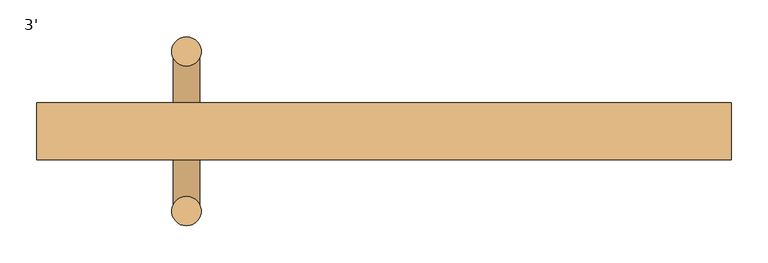
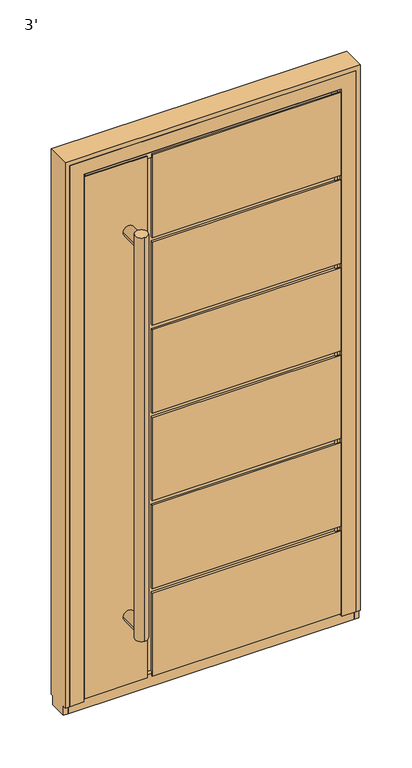
"""IFC4 building model written with IfcOpenShell, lengths in millimetres: door geometry, 3'."""

from ifc_helpers import new_model, si_unit, point, frame, frame_2d, origin, place, context, project, spatial, circle_curve, trimmed, segment, composite_curve, outline, extrude, faceted_brep, source, transform, mapped, element, save


def door_3_44036f4b(model_context):
    return source(origin(), model_context, "Body", "SolidModel", [
        extrude(outline(composite_curve([segment(trimmed(circle_curve(frame_2d((-268.65, 90.8003001)), 20.0), [point((-268.65, 70.8003001))], [point((-268.65, 110.8003001))], False, "CARTESIAN"), True, "CONTINUOUS"), segment(trimmed(circle_curve(frame_2d((-268.65, 90.8003001)), 20.0), [point((-268.65, 110.8003001))], [point((-268.65, 70.8003001))], False, "CARTESIAN"), True, "CONTINUOUS")], self_intersect=False)), frame((0.0, 0.0, 210.0000003), z_axis=(0.0, 0.0, 1.0), x_axis=(1.0, 0.0, 0.0)), (0.0, 0.0, 1.0), 1363.8),
        extrude(outline(composite_curve([segment(trimmed(circle_curve(frame_2d((-268.65, -126.2003001)), 20.0), [point((-268.65, -146.2003001))], [point((-268.65, -106.2003001))], False, "CARTESIAN"), True, "CONTINUOUS"), segment(trimmed(circle_curve(frame_2d((-268.65, -126.2003001)), 20.0), [point((-268.65, -106.2003001))], [point((-268.65, -146.2003001))], False, "CARTESIAN"), True, "CONTINUOUS")], self_intersect=False)), frame((0.0, 0.0, 210.0000003), z_axis=(0.0, 0.0, 1.0), x_axis=(1.0, 0.0, 0.0)), (0.0, 0.0, 1.0), 1363.8),
        extrude(outline(composite_curve([segment(trimmed(circle_curve(frame_2d((241.9000003, -268.65)), 18.0), [point((241.9000003, -286.65))], [point((241.9000003, -250.65))], False, "CARTESIAN"), True, "CONTINUOUS"), segment(trimmed(circle_curve(frame_2d((241.9000003, -268.65)), 18.0), [point((241.9000003, -250.65))], [point((241.9000003, -286.65))], False, "CARTESIAN"), True, "CONTINUOUS")], self_intersect=False)), frame((0.0, -126.2, 0.0), z_axis=(0.0, 1.0, 0.0), x_axis=(0.0, 0.0, 1.0)), (0.0, 0.0, 1.0), 217.0),
        extrude(outline(composite_curve([segment(trimmed(circle_curve(frame_2d((1541.9000003, -268.65)), 18.0), [point((1541.9000003, -286.65))], [point((1541.9000003, -250.65))], False, "CARTESIAN"), True, "CONTINUOUS"), segment(trimmed(circle_curve(frame_2d((1541.9000003, -268.65)), 18.0), [point((1541.9000003, -250.65))], [point((1541.9000003, -286.65))], False, "CARTESIAN"), True, "CONTINUOUS")], self_intersect=False)), frame((0.0, -126.2, 0.0), z_axis=(0.0, 1.0, 0.0), x_axis=(0.0, 0.0, 1.0)), (0.0, 0.0, 1.0), 217.0),
        faceted_brep([(-193.65, 13.8, 306.466667), (383.65, 13.8, 306.466667), (383.65, 13.8, 291.466667), (-193.65, 13.8, 291.466667), (-193.65, 13.8, 35.0), (-208.65, 13.8, 35.0), (-208.65, 13.8, 1748.8000003), (-193.65, 13.8, 1748.8000003), (-193.65, 13.8, 1492.3333337), (383.65, 13.8, 1492.3333337), (383.65, 13.8, 1477.3333337), (-193.65, 13.8, 1477.3333337), (-193.65, 13.8, 1195.866667), (383.65, 13.8, 1195.866667), (383.65, 13.8, 1180.866667), (-193.65, 13.8, 1180.866667), (-193.65, 13.8, 899.4000004), (383.65, 13.8, 899.4000004), (383.65, 13.8, 884.4000004), (-193.65, 13.8, 884.4000004), (-193.65, 13.8, 602.9333337), (383.65, 13.8, 602.9333337), (383.65, 13.8, 587.9333337), (-193.65, 13.8, 587.9333337), (-193.65, 20.8, 587.9333337), (-193.65, 20.8, 306.466667), (383.65, 20.8, 587.9333337), (383.65, 11.7997698, 1748.8000003), (383.65, 11.7997698, 35.0), (383.65, 18.8020472, 35.0), (383.65, 18.8020472, 24.0), (383.65, 20.8, 24.0), (383.65, 20.8, 291.466667), (383.65, 20.8, 306.466667), (383.65, 20.8, 602.9333337), (383.65, 20.8, 884.4000004), (383.65, 20.8, 899.4000004), (383.65, 20.8, 1180.866667), (383.65, 20.8, 1195.866667), (383.65, 20.8, 1477.3333337), (383.65, 20.8, 1492.3333337), (383.65, 20.8, 1748.8000003), (-193.65, 20.8, 602.9333337), (-193.65, 20.8, 884.4000004), (-193.65, 20.8, 899.4000004), (-193.65, 20.8, 1180.866667), (-208.65, 18.8020472, 35.0), (-208.65, 18.8020472, 24.0), (-208.65, 20.8, 24.0), (-208.65, 20.8, 1748.8000003), (-383.65, 11.7997698, 35.0), (-383.65, 18.8020472, 35.0), (-193.65, 18.8020472, 35.0), (-193.65, 20.8, 291.466667), (-193.65, 20.8, 24.0), (-193.65, 18.8020472, 24.0), (-383.65, 18.8020472, 24.0), (-383.65, 20.8, 24.0), (-383.65, 20.8, 1748.8000003), (-193.65, 20.8, 1195.866667), (-193.65, 20.8, 1477.3333337), (-193.65, 20.8, 1492.3333337), (-193.65, 20.8, 1748.8000003), (408.65, -56.2, 10.0000003), (-193.65, -56.2, 10.0000003), (-193.65, -53.2, 10.0000003), (408.65, -53.2, 10.0000003), (-408.65, -53.2, 10.0000003), (-208.65, -53.2, 10.0000003), (-208.65, -56.2, 10.0000003), (-408.65, -56.2, 10.0000003), (408.65, -56.2, 306.466667), (408.65, -53.2, 306.466667), (408.65, -53.2, 587.9333337), (408.65, -56.2, 587.9333337), (408.65, -56.2, 899.4000004), (408.65, -53.2, 899.4000004), (408.65, -53.2, 1180.866667), (408.65, -56.2, 1180.866667), (408.65, -56.2, 602.9333337), (408.65, -53.2, 602.9333337), (408.65, -53.2, 884.4000004), (408.65, -56.2, 884.4000004), (408.65, -56.2, 1195.866667), (408.65, -53.2, 1195.866667), (408.65, -53.2, 1477.3333337), (408.65, -56.2, 1477.3333337), (408.65, -56.2, 1773.8000003), (408.65, -56.2, 1492.3333337), (408.65, -53.2, 1492.3333337), (408.65, -53.2, 1773.8000003), (408.65, -53.2, 291.466667), (408.65, -56.2, 291.466667), (-193.65, -53.2, 25.5), (393.15, -53.2, 25.5), (393.15, -53.2, 291.466667), (393.15, -53.2, 306.466667), (393.15, -53.2, 587.9333337), (393.15, -53.2, 899.4000004), (393.15, -53.2, 1180.866667), (393.15, -53.2, 602.9333337), (393.15, -53.2, 884.4000004), (-393.15, -53.2, 25.5), (-208.65, -53.2, 25.5), (-408.65, -53.2, 1773.8000003), (-208.65, -53.2, 1773.8000003), (-208.65, -53.2, 1758.3000003), (-393.15, -53.2, 1758.3000003), (393.15, -53.2, 1195.866667), (393.15, -53.2, 1477.3333337), (393.15, -53.2, 1492.3333337), (393.15, -53.2, 1758.3000003), (-193.65, -53.2, 1758.3000003), (-193.65, -53.2, 1773.8000003), (-193.65, -49.2, 291.466667), (-193.65, -49.2, 25.5), (-193.65, -56.2, 291.466667), (-208.65, -56.2, 1773.8000003), (-408.65, -56.2, 1773.8000003), (-193.65, -56.2, 587.9333337), (-193.65, -56.2, 306.466667), (-193.65, -56.2, 1180.866667), (-193.65, -56.2, 899.4000004), (-193.65, -56.2, 884.4000004), (-193.65, -56.2, 602.9333337), (-193.65, -56.2, 1477.3333337), (-193.65, -56.2, 1195.866667), (-193.65, -56.2, 1773.8000003), (-193.65, -56.2, 1492.3333337), (-208.65, -49.2, 1758.3000003), (-208.65, -49.2, 25.5), (-383.65, 11.7997698, 1748.8000003), (393.15, 11.7997698, 1758.3000003), (393.15, 11.7997698, 25.5), (-393.15, 11.7997698, 25.5), (-393.15, 11.7997698, 1758.3000003), (393.15, -49.2, 1492.3333337), (393.15, -49.2, 1477.3333337), (393.15, -49.2, 1195.866667), (393.15, -49.2, 1180.866667), (393.15, -49.2, 899.4000004), (393.15, -49.2, 884.4000004), (393.15, -49.2, 602.9333337), (393.15, -49.2, 587.9333337), (393.15, -49.2, 306.466667), (393.15, -49.2, 291.466667), (-193.65, -49.2, 1477.3333337), (-193.65, -49.2, 1492.3333337), (-193.65, -49.2, 1758.3000003), (-193.65, -49.2, 306.466667), (-193.65, -49.2, 587.9333337), (-193.65, -49.2, 602.9333337), (-193.65, -49.2, 884.4000004), (-193.65, -49.2, 899.4000004), (-193.65, -49.2, 1180.866667), (-193.65, -49.2, 1195.866667)], [[[0, 1, 2, 3, 4, 5, 6, 7, 8, 9, 10, 11, 12, 13, 14, 15, 16, 17, 18, 19, 20, 21, 22, 23]], [[23, 24, 25, 0]], [[23, 22, 26, 24]], [[27, 28, 29, 30, 31, 32, 2, 1, 33, 26, 22, 21, 34, 35, 18, 17, 36, 37, 14, 13, 38, 39, 10, 9, 40, 41]], [[42, 34, 21, 20]], [[19, 43, 42, 20]], [[19, 18, 35, 43]], [[44, 36, 17, 16]], [[15, 45, 44, 16]], [[5, 46, 47, 48, 49, 6]], [[28, 50, 51, 46, 5, 4, 52, 29]], [[53, 54, 55, 52, 4, 3]], [[3, 2, 32, 53]], [[25, 33, 1, 0]], [[29, 52, 55, 30]], [[56, 47, 46, 51]], [[30, 55, 54, 31]], [[57, 48, 47, 56]], [[36, 44, 45, 37]], [[34, 42, 43, 35]], [[33, 25, 24, 26]], [[54, 53, 32, 31]], [[58, 49, 48, 57]], [[38, 59, 60, 39]], [[41, 40, 61, 62]], [[63, 64, 65, 66]], [[67, 68, 69, 70]], [[71, 72, 73, 74]], [[75, 76, 77, 78]], [[79, 80, 81, 82]], [[83, 84, 85, 86]], [[87, 88, 89, 90]], [[66, 91, 92, 63]], [[65, 93, 94, 95, 91, 66]], [[72, 96, 97, 73]], [[76, 98, 99, 77]], [[80, 100, 101, 81]], [[102, 103, 68, 67, 104, 105, 106, 107]], [[84, 108, 109, 85]], [[90, 89, 110, 111, 112, 113]], [[114, 115, 93, 65, 64, 116]], [[70, 69, 117, 118]], [[63, 92, 116, 64]], [[74, 119, 120, 71]], [[78, 121, 122, 75]], [[82, 123, 124, 79]], [[86, 125, 126, 83]], [[87, 127, 128, 88]], [[70, 118, 104, 67]], [[129, 106, 105, 117, 69, 68, 103, 130]], [[58, 57, 56, 51, 50, 131]], [[132, 133, 134, 135], [131, 50, 28, 27]], [[111, 110, 136, 137, 109, 108, 138, 139, 99, 98, 140, 141, 101, 100, 142, 143, 97, 96, 144, 145, 95, 94, 133, 132]], [[94, 93, 115, 130, 103, 102, 134, 133]], [[135, 134, 102, 107]], [[146, 137, 136, 147, 148, 129, 130, 115, 114, 145, 144, 149, 150, 143, 142, 151, 152, 141, 140, 153, 154, 139, 138, 155]], [[153, 122, 121, 154]], [[153, 140, 98, 76, 75, 122]], [[123, 82, 81, 101, 141, 152]], [[151, 124, 123, 152]], [[151, 142, 100, 80, 79, 124]], [[119, 74, 73, 97, 143, 150]], [[149, 120, 119, 150]], [[149, 144, 96, 72, 71, 120]], [[116, 92, 91, 95, 145, 114]], [[15, 14, 37, 45]], [[59, 38, 13, 12]], [[11, 60, 59, 12]], [[11, 10, 39, 60]], [[61, 40, 9, 8]], [[8, 7, 62, 61]], [[125, 86, 85, 109, 137, 146]], [[128, 127, 113, 112, 148, 147]], [[121, 78, 77, 99, 139, 154]], [[155, 138, 108, 84, 83, 126]], [[155, 126, 125, 146]], [[147, 136, 110, 89, 88, 128]], [[90, 113, 127, 87]], [[118, 117, 105, 104]], [[132, 135, 107, 106, 129, 148, 112, 111]], [[27, 41, 62, 7, 6, 49, 58, 131]]]),
        faceted_brep([(-457.2, -56.2, 0.0), (-457.2, -47.1997571, 0.0), (-412.7, -47.1997571, 0.0), (-412.7, -56.2, 0.0), (-403.2, 16.2999958, 0.0), (-403.2, 11.8, 0.0), (-457.2, 11.8, 0.0), (-457.2, 20.8, 0.0), (-387.7, 20.8, 0.0), (-387.7, 16.2999958, 0.0), (457.2, 20.8, 0.0), (457.2, 11.8, 0.0), (403.2, 11.8, 0.0), (403.2, 16.2999958, 0.0), (387.7, 16.2999958, 0.0), (387.7, 20.8, 0.0), (412.7, -47.1997571, 0.0), (457.2, -47.1997571, 0.0), (457.2, -56.2, 0.0), (412.7, -56.2, 0.0), (-457.2, 11.8, -30.0), (-457.2, -47.1997571, -30.0), (-457.2, -56.2, 1828.8), (-457.2, 20.8, 1828.8), (-412.7, -56.2, 1784.3), (412.7, -56.2, 1784.3), (457.2, -56.2, 1828.8), (457.2, 20.8, 1828.8), (457.2, -47.1997571, -30.0), (457.2, 11.8, -30.0), (387.7, 20.8, 1759.3), (-387.7, 20.8, 1759.3), (-403.2, -47.2, 1774.8), (-403.2, -47.2, 14.5), (-403.2, 11.8, 14.5), (-403.2, 16.2999958, 1774.8), (403.2, 16.2999958, 1774.8), (403.2, -47.2, 1774.8), (403.2, 11.8, 14.5), (403.2, -47.2, 14.5), (-412.7, -47.2, 1784.3), (412.7, -47.2, 1784.3), (-387.7, 16.2999958, 1759.3), (387.7, 16.2999958, 1759.3)], [[[0, 1, 2, 3]], [[4, 5, 6, 7, 8, 9]], [[10, 11, 12, 13, 14, 15]], [[16, 17, 18, 19]], [[7, 6, 20, 21, 1, 0, 22, 23]], [[3, 24, 25, 19, 18, 26, 22, 0]], [[22, 26, 27, 23]], [[18, 17, 28, 29, 11, 10, 27, 26]], [[7, 23, 27, 10, 15, 30, 31, 8]], [[32, 33, 34, 5, 4, 35]], [[35, 36, 37, 32]], [[36, 13, 12, 38, 39, 37]], [[40, 24, 3, 2]], [[16, 41, 40, 2, 1, 21, 28, 17], [37, 39, 33, 32]], [[9, 42, 43, 14, 13, 36, 35, 4]], [[8, 31, 42, 9]], [[24, 40, 41, 25]], [[30, 43, 42, 31]], [[19, 25, 41, 16]], [[14, 43, 30, 15]], [[20, 6, 5, 34, 38, 12, 11, 29]], [[39, 38, 34, 33]], [[20, 29, 28, 21]]]),
        faceted_brep([(-457.2, -47.2, -30.0), (-472.2, -47.2, -30.0), (-472.2, 11.8, -30.0), (-457.2, 11.8, -30.0), (-457.2, -56.2, 1828.8), (-457.2, -56.2, 0.0), (-457.2, -47.2, 0.0), (-457.2, 11.8, 0.0), (-457.2, 20.8, 0.0), (-457.2, 20.8, 1828.8), (-472.2, 11.8, 0.0), (472.2, 11.8, 0.0), (472.2, 11.8, -30.0), (457.2, 11.8, -30.0), (457.2, 11.8, 0.0), (-472.2, 20.8, 1843.8), (-472.2, 20.8, 0.0), (-472.2, -47.2, 0.0), (-472.2, -56.2, 0.0), (-472.2, -56.2, 1843.8), (457.2, -47.2, 0.0), (457.2, -47.2, -30.0), (472.2, -47.2, -30.0), (472.2, -47.2, 0.0), (457.2, 20.8, 1828.8), (457.2, 20.8, 0.0), (457.2, -56.2, 0.0), (457.2, -56.2, 1828.8), (472.2, -56.2, 0.0), (472.2, -56.2, 1843.8), (472.2, 20.8, 0.0), (472.2, 20.8, 1843.8)], [[[0, 1, 2, 3]], [[4, 5, 6, 0, 3, 7, 8, 9]], [[7, 3, 2, 10]], [[11, 12, 13, 14]], [[15, 16, 10, 2, 1, 17, 18, 19]], [[17, 1, 0, 6]], [[20, 21, 22, 23]], [[24, 25, 14, 13, 21, 20, 26, 27]], [[27, 26, 28, 29, 19, 18, 5, 4]], [[6, 5, 18, 17]], [[23, 28, 26, 20]], [[22, 21, 13, 12]], [[10, 16, 8, 7]], [[14, 25, 30, 11]], [[9, 8, 16, 15, 31, 30, 25, 24]], [[29, 28, 23, 22, 12, 11, 30, 31]], [[9, 24, 27, 4]], [[19, 29, 31, 15]]]),
    ])


if __name__ == "__main__":
    model = new_model("IFC4")
    model_context = context("Model", 3, world=origin())
    ifc_project = project(units=[si_unit("LENGTHUNIT", "METRE", prefix="MILLI")], contexts=[model_context])
    site = spatial("IfcSite", under=ifc_project)
    building = spatial("IfcBuilding", under=site)
    placement = place(None, origin())
    door_3_shape = door_3_44036f4b(model_context)
    element("IfcDoor", 1, ObjectType="3'", at=placement, inside=building, context=model_context, shape_type="MappedRepresentation", body=[
        mapped(door_3_shape, transform((0.0, 0.0, 0.0), x_axis=(1.0, 0.0, 0.0), y_axis=(0.0, 1.0, 0.0), z_axis=(0.0, 0.0, 1.0))),
    ])
    save(model, "model.ifc")

# Revit data of these elements
# Type "3'"
#   Type Mark = "9"
#   Water resistance = "up to Class E900, EN 12208:2001"
#   Uniclass2015Version = "v1.21"
#   Uniclass2015Reference = "Ss_25_30_20_30"
#   Uniclass2015Description = "Frame and door leaf system"
#   URL = "www.aluprof.com"
#   Type IFC Predefined Type = "USERDEFINED"
#   Right-hand / Left-hand door [instance default] = ""
#   Resistance to wind load = "up to Class C5/B5, EN 12210:2001"
#   Insert type = "ST"
#   Hardware [instance default] = ""
#   Product page = "https://aluprof.com/en/architects/offer/window-and-door-systems/panel-doors#visualisation"
#   Operation = "SinglePanelOutwardOpening"
#   Opening type = "Outward"
#   NBSReference = "25-50-20/125"
#   NBSDescription = "Frame and door leaf system"
#   Important = "The actual acceptable construction dimensions are dependent on the selection of profiles and hardware, glazing type, construction weight and the construction’s operating conditions. These should be determined by a suitably qualified person, and using ALUPROF’s calculation software"
#   IfcExportType = "USERDEFINED"
#   IfcExportAs = "IfcDoorType"
#   Handle type [instance default] = ""
#   Manufacturer = "ALUPROF SA"
#   Export Type to IFC As = "IfcDoorType"
#   Door sill type [instance default] = ""
#   Description = "External single-leaf panel door outward opening"
#   Model = "MB-86 ST Panel Door AD07"
#   Content of the recyclate in the material = "69.2%"
#   COBie.Type.WarrantyDurationParts = ""
#   COBie.Type.Name = ""
#   COBie.Type.Manufacturer = "ALUPROF SA"
#   COBie.Space.Name = ""
#   COBie.Floor.Name = ""
#   COBie.Facility.Name = ""
#   COBie.CreatedOn = ""
#   COBie.Component.WarrantyStartDate = ""
#   COBie.Component.Name = "MB-86 ST Panel Door AD07"
#   Burglar resistance = "RC2"
#   Air permeability = "up to Class 4, EN 12207:2001"
#   Width of the active leaf = 2' - 8.17717"
#   Placement in wall = 0' - 0.7874"
#   Thickness = 0' - 3.0315"
#   Height of the opening sash = 5' - 9.44094"
#   Handle Offset = 3' - 5.33858"
#   Rough Height = 6' - 2.40945"
#   Rough Width = 3' - 1.1811"
#   Height = 6' - 0"
#   Width = 3' - 0"
#   Construction depth = 0' - 3.0315"
#   Clear opening width = 2' - 3.94882"
#   Clear opening height = 5' - 8.47638"
#   Height of the array = 0' - 11.08136"
#   Schedule No. [instance default] = 1
#   Handrail [instance default] = yes
#   IsExternal = yes
#   Handle [instance default] = no
#   Door closer [instance default] = no
#   Function = 1
#   COBie.Type = yes
#   COBie = yes
#   Access control [instance default] = no
#   Panel = element 380783
#   Wall Closure = (empty or 0)
